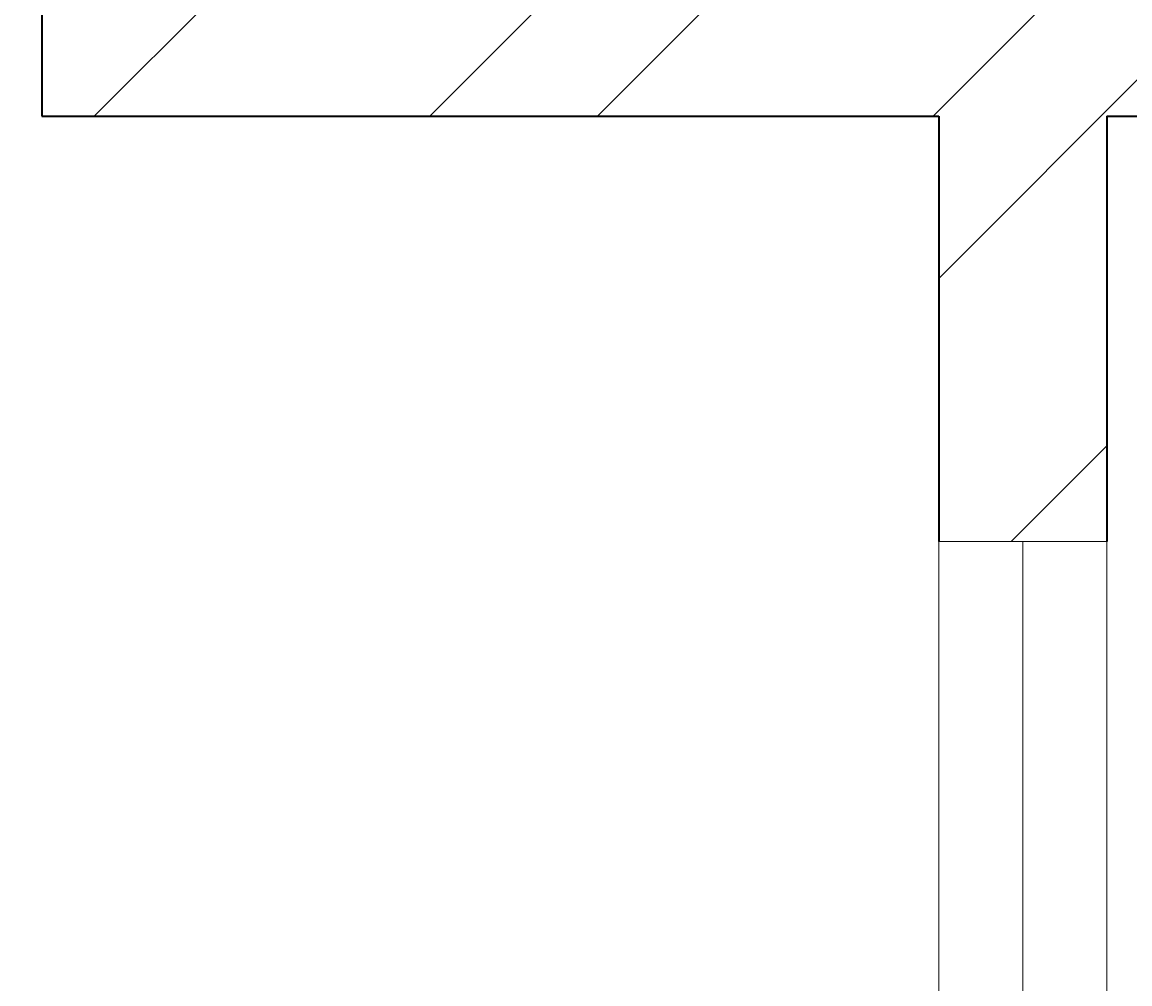
# Model space of a CAD drawing. Units: inches. Extents: x 1885 to 2748, y 783 to 2421.
# Tile 69 of 117: x 1992 to 2022, y 2047 to 2073. Entities that reach past the tile are written whole.
import ezdxf

# ---------------------------------------------------------------- set-up
doc = ezdxf.new("R2010")
doc.units = ezdxf.units.IN
for name, color, linetype, lineweight in [('A-ANNO-DIMS', 2, 'Continuous', 18), ('A-GLAZ', 181, 'Continuous', 18), ('A-WALL', 7, 'Continuous', 35)]:
    doc.layers.add(name, color=color, linetype=linetype, lineweight=lineweight)
doc.layers.add('A-WALL-PATT', color=85, linetype='Continuous', lineweight=13, true_color=0x58ba48)
doc.styles.get("Standard").update_dxf_attribs({"font": 'arial.ttf'})
doc.dimstyles.get("Standard").update_dxf_attribs({"dimtxt": 0.18, "dimasz": 0.18, "dimexe": 0.18, "dimexo": 0.0625, "dimgap": 0.09, "dimtad": 0, "dimtih": 1, "dimtoh": 1, "dimdec": 4, "dimzin": 0, "dimdsep": 46, "dimtxsty": 'Standard', "dimcen": 0.09, "dimadec": 0, "dimazin": 0, "dimtfac": 1, "dimtdec": 4, "dimtofl": 0, "dimtmove": 0, "dimatfit": 3, "dimfxl": 1, "dimtolj": 1, "dimtzin": 0, "dimarcsym": 0})

# ---------------------------------------------------------------- blocks, each defined once
blk = doc.blocks.new('*D48')
at = {"layer": 'A-ANNO-DIMS', "color": 0, "lineweight": -2, "transparency": 16777216}
for p, q in [((1980.711, 2348.006), (1902.844, 2348.006)), ((1903.024, 2347.826), (1903.024, 2114.937)), ((1903.024, 1881.686), (1903.024, 2114.574)), ((2016.711, 1881.506), (1902.844, 1881.506))]:
    blk.add_line(p, q, dxfattribs=at)
at = {"layer": 'A-ANNO-DIMS', "color": 0, "transparency": 16777216}
for points in [[(1902.994, 2347.826), (1903.054, 2347.826), (1903.024, 2348.006)], [(1902.994, 1881.686), (1903.054, 1881.686), (1903.024, 1881.506)]]:
    blk.add_solid(points, dxfattribs=at)
at = {"layer": 'Defpoints', "color": 0, "transparency": 16777216}
for p in [(1903.024, 2348.006), (1980.774, 2348.006), (2016.774, 1881.506)]:
    blk.add_point(p, dxfattribs=at)
at = {"layer": 'A-ANNO-DIMS', "color": 0, "transparency": 16777216, "insert": (1903.024, 2114.756), "char_height": 0.18, "attachment_point": 5}
blk.add_mtext('\\A1;466.5', dxfattribs=at)

msp = doc.modelspace()

# ---------------------------------------------------------------- hatches: boundary and pattern name
at = {"layer": 'A-WALL-PATT'}
h = msp.add_hatch(dxfattribs=at)
h.set_pattern_fill('ANSI32', color=256)
h.paths.add_polyline_path([(2007.772, 2318.006), (1980.774, 2318.006), (1980.774, 2281.215), (1985.274, 2281.215), (1985.274, 2313.506), (2007.772, 2313.506), (2007.772, 2315.756)])
h.paths.add_polyline_path([(2094.324, 2318.006), (2067.772, 2318.006), (2067.772, 2313.506), (2094.324, 2313.506), (2094.324, 2315.756)])
h.paths.add_polyline_path([(2131.367, 2315.756), (2131.367, 2318.006), (2131.189, 2318.006), (2112.609, 2318.006), (2112.609, 2313.506), (2117.274, 2313.506), (2117.274, 2255.201), (2121.774, 2255.201), (2121.774, 2313.506), (2131.367, 2313.506)])
h.paths.add_polyline_path([(2190.512, 2318.006), (2155.367, 2318.006), (2155.367, 2313.506), (2169.774, 2313.506), (2169.774, 2229.506), (2121.774, 2229.506), (2121.774, 2233.451), (2119.524, 2233.451), (2117.274, 2233.451), (2117.274, 2201.101), (2121.774, 2201.101), (2121.774, 2225.006), (2169.774, 2225.006), (2169.774, 2165.006), (2306.274, 2165.006), (2306.274, 2066.006), (2310.774, 2066.006), (2344.274, 2066.006), (2486.274, 2066.006), (2486.274, 1886.006), (2483.02, 1886.006), (2483.02, 1881.506), (2486.274, 1881.506), (2486.274, 1880.678), (2490.774, 1880.678), (2490.774, 2070.506), (2344.274, 2070.506), (2310.774, 2070.506), (2310.774, 2165.006), (2310.774, 2173.636), (2308.524, 2173.636), (2306.274, 2173.636), (2306.274, 2169.506), (2174.274, 2169.506), (2174.274, 2313.506), (2190.512, 2313.506), (2190.512, 2315.756)])
h.paths.add_polyline_path([(1985.274, 2221.215), (1980.774, 2221.215), (1980.774, 2165.006), (1992.774, 2165.006), (1992.774, 2141.927), (1997.274, 2141.927), (1997.274, 2165.006), (2117.274, 2165.006), (2117.274, 2163.126), (2121.774, 2163.126), (2121.774, 2172.734), (2119.524, 2172.734), (2117.274, 2172.734), (2117.274, 2169.506), (1985.274, 2169.506)])
h.paths.add_polyline_path([(1997.274, 2105.927), (1992.774, 2105.927), (1992.774, 2070.506), (2016.774, 2070.506), (2016.774, 2059.123), (2019.024, 2059.123), (2021.274, 2059.123), (2021.274, 2070.506), (2117.274, 2070.506), (2117.274, 2022.506), (2114.423, 2022.506), (2114.423, 2018.006), (2123.627, 2018.006), (2123.627, 2020.256), (2123.627, 2022.506), (2121.774, 2022.506), (2121.774, 2142.587), (2119.524, 2142.587), (2117.274, 2142.587), (2117.274, 2075.006), (1997.274, 2075.006)])
h.paths.add_polyline_path([(2092.029, 2020.256), (2092.029, 2022.506), (2021.274, 2022.506), (2021.274, 2035.123), (2016.774, 2035.123), (2016.774, 2018.006), (2016.774, 1978.784), (2021.274, 1978.784), (2021.274, 2018.006), (2092.029, 2018.006)])
h.paths.add_polyline_path([(2260.938, 2022.506), (2153.105, 2022.506), (2153.105, 2020.256), (2153.105, 2018.006), (2155.274, 2018.006), (2155.274, 1886.006), (2107.629, 1886.006), (2107.629, 1881.506), (2182.911, 1881.506), (2182.911, 1883.756), (2182.911, 1886.006), (2159.774, 1886.006), (2159.774, 2018.006), (2260.938, 2018.006), (2260.938, 2020.256)])
h.paths.add_polyline_path([(2047.629, 1883.756), (2047.629, 1886.006), (2021.274, 1886.006), (2021.274, 1918.784), (2019.024, 1918.784), (2016.774, 1918.784), (2016.774, 1881.506), (2047.629, 1881.506)])
h.paths.add_polyline_path([(2306.361, 1883.756), (2306.361, 1886.006), (2296.274, 1886.006), (2296.274, 1982.006), (2316.535, 1982.006), (2316.535, 1984.256), (2316.535, 1986.506), (2296.274, 1986.506), (2296.274, 2022.506), (2289.276, 2022.506), (2289.276, 2018.006), (2291.774, 2018.006), (2291.774, 1886.006), (2242.911, 1886.006), (2242.911, 1881.506), (2306.361, 1881.506)], flags=17)
h.paths.add_polyline_path([(1985.274, 1843.006), (2021.6, 1843.006), (2021.534, 1845.441), (2021.477, 1847.506), (1980.774, 1847.506), (1980.774, 1809.446), (1985.274, 1809.446)])
h.paths.add_polyline_path([(2131.482, 1845.256), (2131.482, 1847.506), (2081.534, 1847.506), (2081.534, 1843.006), (2117.274, 1843.006), (2117.274, 1784.147), (2119.524, 1784.147), (2121.774, 1784.147), (2121.774, 1843.006), (2131.482, 1843.006)])
h.paths.add_polyline_path([(2203.886, 1847.506), (2155.482, 1847.506), (2155.482, 1843.006), (2169.774, 1843.006), (2169.774, 1759.006), (2121.774, 1759.006), (2121.774, 1761.457), (2117.274, 1761.457), (2117.274, 1730.429), (2121.774, 1730.429), (2121.774, 1754.506), (2177.421, 1754.506), (2177.421, 1756.756), (2177.421, 1759.006), (2174.274, 1759.006), (2174.274, 1843.006), (2203.886, 1843.006)])
h.paths.add_polyline_path([(2335.554, 1845.256), (2335.554, 1847.506), (2239.886, 1847.506), (2239.886, 1843.006), (2306.274, 1843.006), (2306.274, 1759.006), (2199.486, 1759.006), (2199.486, 1754.506), (2310.774, 1754.506), (2310.774, 1843.006), (2335.554, 1843.006)])
h.paths.add_polyline_path([(2348.774, 2022.506), (2344.274, 2022.506), (2344.274, 1986.506), (2341.681, 1986.506), (2341.681, 1982.006), (2344.274, 1982.006), (2344.274, 1886.006), (2330.361, 1886.006), (2330.361, 1881.506), (2361.627, 1881.506), (2361.627, 1883.756), (2361.627, 1886.006), (2348.774, 1886.006)], flags=17)
h.paths.add_polyline_path([(2283.251, 2315.756), (2283.251, 2318.006), (2238.512, 2318.006), (2238.512, 2313.506), (2283.251, 2313.506)], flags=17)
h.paths.add_polyline_path([(2363.274, 2348.006), (2388.677, 2348.006), (2388.677, 2350.256), (2388.677, 2352.506), (2358.774, 2352.506), (2358.774, 2348.006), (2358.774, 2318.006), (2344.481, 2318.006), (2344.481, 2313.506), (2358.774, 2313.506), (2358.774, 2229.506), (2310.774, 2229.506), (2310.774, 2231.952), (2306.274, 2231.952), (2306.274, 2205.611), (2310.774, 2205.611), (2310.774, 2225.006), (2358.774, 2225.006), (2358.774, 2211.506), (2452.329, 2211.506), (2452.329, 2213.756), (2452.329, 2216.006), (2363.274, 2216.006), (2363.274, 2318.006)])
h.paths.add_polyline_path([(2310.774, 2313.506), (2320.481, 2313.506), (2320.481, 2315.756), (2320.481, 2318.006), (2302.728, 2318.006), (2302.728, 2313.506), (2306.274, 2313.506), (2306.274, 2251.076), (2310.774, 2251.076)], flags=17)
h.paths.add_polyline_path([(2490.774, 2352.506), (2486.274, 2352.506), (2448.677, 2352.506), (2448.677, 2348.006), (2486.274, 2348.006), (2486.274, 2318.006), (2486.274, 2216.006), (2481.78, 2216.006), (2481.78, 2211.506), (2486.274, 2211.506), (2486.274, 2165.006), (2493.289, 2165.006), (2493.289, 2167.256), (2493.289, 2169.506), (2490.774, 2169.506), (2490.774, 2313.506), (2494.429, 2313.506), (2494.429, 2318.006), (2490.774, 2318.006)])
h.paths.add_polyline_path([(2534.653, 2318.006), (2515.691, 2318.006), (2515.691, 2313.506), (2534.653, 2313.506), (2534.653, 2315.756)])
h.paths.add_polyline_path([(2618.274, 2318.006), (2594.653, 2318.006), (2594.653, 2313.506), (2613.774, 2313.506), (2613.774, 2281.706), (2618.274, 2281.706)])
h.paths.add_polyline_path([(2618.274, 2221.706), (2613.774, 2221.706), (2613.774, 2169.506), (2554.019, 2169.506), (2554.019, 2165.006), (2613.774, 2165.006), (2613.774, 2152.878), (2618.274, 2152.878)])
h.paths.add_polyline_path([(2618.274, 2128.878), (2616.024, 2128.878), (2613.774, 2128.878), (2613.774, 2117.006), (2529.774, 2117.006), (2529.774, 2165.006), (2532.848, 2165.006), (2532.848, 2169.506), (2522.867, 2169.506), (2522.867, 2165.006), (2525.274, 2165.006), (2525.274, 2117.006), (2525.274, 2112.506), (2525.274, 2108.576), (2529.774, 2108.576), (2529.774, 2112.506), (2613.774, 2112.506), (2613.774, 2080.19), (2618.274, 2080.19)])
h.paths.add_polyline_path([(2618.274, 2044.19), (2616.024, 2044.19), (2613.774, 2044.19), (2613.774, 2015.506), (2529.774, 2015.506), (2529.774, 2088.582), (2527.524, 2088.582), (2525.274, 2088.582), (2525.274, 2011.006), (2613.774, 2011.006), (2613.774, 1956.755), (2618.274, 1956.755)])
h.paths.add_polyline_path([(2618.274, 1881.506), (2618.274, 1896.755), (2613.774, 1896.755), (2613.774, 1881.506), (2613.774, 1847.506), (2592.715, 1847.506), (2592.715, 1843.006), (2613.774, 1843.006), (2613.774, 1765.006), (2613.774, 1760.506), (2609.621, 1760.506), (2609.621, 1756.006), (2613.774, 1756.006), (2613.774, 1660.006), (2608.544, 1660.006), (2608.544, 1655.506), (2613.774, 1655.506), (2613.774, 1508.158), (2618.274, 1508.158)])
h.paths.add_polyline_path([(2565.774, 1843.006), (2568.997, 1843.006), (2568.997, 1847.506), (2490.774, 1847.506), (2490.774, 1849.7), (2488.524, 1849.7), (2486.274, 1849.7), (2486.274, 1847.506), (2477.274, 1847.506), (2477.274, 1838.506), (2477.274, 1821.493), (2486.274, 1821.493), (2486.274, 1838.506), (2561.274, 1838.506), (2561.274, 1765.006), (2486.274, 1765.006), (2486.274, 1786.157), (2477.274, 1786.157), (2477.274, 1765.006), (2477.274, 1756.006), (2486.274, 1756.006), (2565.774, 1756.006), (2585.621, 1756.006), (2585.621, 1758.256), (2585.621, 1760.506), (2565.774, 1760.506), (2565.774, 1765.006)])
h.paths.add_polyline_path([(2486.274, 1651.006), (2561.274, 1651.006), (2561.274, 1567.006), (2486.274, 1567.006), (2486.274, 1591.321), (2477.274, 1591.321), (2477.274, 1567.006), (2477.274, 1558.006), (2477.274, 1555.439), (2481.774, 1555.439), (2481.774, 1558.006), (2568.653, 1558.006), (2568.653, 1560.256), (2568.653, 1562.506), (2565.774, 1562.506), (2565.774, 1655.506), (2584.544, 1655.506), (2584.544, 1657.756), (2584.544, 1660.006), (2565.774, 1660.006), (2486.274, 1660.006), (2477.274, 1660.006), (2477.274, 1651.006), (2477.274, 1632.989), (2486.274, 1632.989)])
h.paths.add_polyline_path([(2449.967, 1883.756), (2449.967, 1886.006), (2421.627, 1886.006), (2421.627, 1881.506), (2449.967, 1881.506)], flags=17)
h.paths.add_polyline_path([(2447.274, 1847.506), (2395.554, 1847.506), (2395.554, 1843.006), (2442.774, 1843.006), (2442.774, 1809.27), (2447.274, 1809.27)])
h.paths.add_polyline_path([(1985.274, 1749.446), (1980.774, 1749.446), (1980.774, 1694.504), (1985.274, 1694.504), (1985.274, 1694.506), (1986.897, 1694.506), (1986.897, 1697.78), (1986.897, 1699.006), (1985.274, 1699.006)])
h.paths.add_polyline_path([(2152.774, 1699.006), (2121.774, 1699.006), (2121.774, 1703.668), (2119.524, 1703.668), (2117.274, 1703.668), (2117.274, 1699.006), (2009.219, 1699.006), (2009.219, 1694.506), (2148.274, 1694.506), (2148.274, 1692.631), (2152.774, 1692.631)])
h.paths.add_polyline_path([(2016.274, 1694.506), (2011.774, 1694.506), (2011.774, 1558.006), (2040.806, 1558.006), (2040.806, 1560.256), (2040.806, 1562.506), (2016.274, 1562.506)])
h.paths.add_polyline_path([(2152.774, 1663.017), (2150.524, 1663.017), (2148.274, 1663.017), (2148.274, 1562.506), (2100.806, 1562.506), (2100.806, 1558.006), (2165.119, 1558.006), (2165.119, 1560.256), (2165.119, 1562.506), (2152.774, 1562.506), (2152.774, 1610.506), (2224.774, 1610.506), (2224.774, 1607.99), (2229.274, 1607.99), (2229.274, 1615.006), (2152.774, 1615.006)])
h.paths.add_polyline_path([(2238.613, 1560.256), (2238.613, 1562.506), (2229.274, 1562.506), (2229.274, 1588.756), (2227.024, 1588.763), (2224.774, 1588.771), (2224.774, 1562.506), (2189.119, 1562.506), (2189.119, 1558.006), (2238.613, 1558.006)])
h.paths.add_polyline_path([(2336.024, 1560.256), (2336.024, 1562.506), (2310.774, 1562.506), (2310.774, 1656.347), (2308.524, 1656.347), (2306.274, 1656.347), (2306.274, 1562.506), (2286.613, 1562.506), (2286.613, 1558.006), (2336.024, 1558.006)])
h.paths.add_polyline_path([(2447.274, 1690.968), (2445.024, 1690.968), (2442.774, 1690.968), (2442.774, 1687.006), (2306.274, 1687.006), (2306.274, 1680.75), (2310.774, 1680.75), (2310.774, 1682.506), (2442.774, 1682.506), (2442.774, 1562.506), (2396.024, 1562.506), (2396.024, 1558.006), (2447.274, 1558.006)])
h.paths.add_polyline_path([(2447.274, 1749.27), (2445.024, 1749.27), (2442.774, 1749.27), (2442.774, 1717.232), (2447.274, 1717.232)])
h.paths.add_polyline_path([(2044.674, 1521.756), (2044.674, 1524.006), (2007.274, 1524.006), (2007.274, 1503.49), (2009.524, 1503.49), (2011.774, 1503.49), (2011.774, 1519.506), (2044.674, 1519.506)])
h.paths.add_polyline_path([(2177.969, 1521.756), (2177.969, 1524.006), (2104.674, 1524.006), (2104.674, 1519.506), (2145.774, 1519.506), (2145.774, 1387.506), (2143.37, 1387.506), (2143.37, 1383.006), (2251.585, 1383.006), (2251.585, 1385.256), (2251.585, 1387.506), (2150.274, 1387.506), (2150.274, 1519.506), (2177.969, 1519.506)])
h.paths.add_polyline_path([(2298.704, 1524.006), (2237.969, 1524.006), (2237.969, 1519.506), (2282.274, 1519.506), (2282.274, 1387.506), (2279.683, 1387.506), (2279.683, 1383.006), (2286.774, 1383.006), (2286.774, 1419.006), (2312.451, 1419.006), (2312.451, 1421.256), (2312.451, 1423.506), (2286.774, 1423.506), (2286.774, 1519.506), (2298.704, 1519.506), (2298.704, 1521.722)], flags=17)
h.paths.add_polyline_path([(2361.897, 1521.756), (2361.897, 1524.006), (2322.704, 1524.006), (2322.704, 1519.506), (2334.774, 1519.506), (2334.774, 1423.506), (2331.93, 1423.506), (2331.93, 1419.006), (2334.774, 1419.006), (2334.774, 1387.506), (2334.774, 1383.228), (2339.274, 1383.228), (2339.274, 1387.506), (2339.274, 1519.506), (2361.897, 1519.506)], flags=17)
h.paths.add_polyline_path([(2447.274, 1521.756), (2447.274, 1524.006), (2421.897, 1524.006), (2421.897, 1519.506), (2447.274, 1519.506)], flags=17)
h.paths.add_polyline_path([(2481.774, 1529.6), (2479.524, 1529.6), (2477.274, 1529.6), (2477.274, 1524.006), (2474.489, 1524.006), (2474.489, 1519.506), (2477.274, 1519.506), (2477.274, 1334.506), (2296.774, 1334.506), (2296.774, 1240.506), (2160.274, 1240.506), (2160.274, 1180.506), (2112.274, 1180.506), (2112.274, 1207.692), (2110.024, 1207.692), (2107.774, 1207.692), (2107.774, 1171.609), (2112.274, 1171.609), (2112.274, 1176.006), (2160.274, 1176.006), (2160.274, 1092.006), (2144.221, 1092.006), (2144.221, 1087.506), (2189.497, 1087.506), (2189.497, 1089.756), (2189.497, 1092.006), (2164.774, 1092.006), (2164.774, 1236.006), (2296.774, 1236.006), (2296.774, 1231.912), (2301.274, 1231.912), (2301.274, 1330.006), (2481.774, 1330.006), (2481.774, 1387.506)])
h.paths.add_polyline_path([(2618.274, 1448.158), (2613.774, 1448.158), (2613.774, 1382.506), (2529.774, 1382.506), (2525.274, 1382.506), (2525.274, 1307.062), (2529.774, 1307.062), (2529.774, 1378.006), (2613.774, 1378.006), (2613.774, 1354.988), (2618.274, 1354.988)])
h.paths.add_polyline_path([(2618.274, 1318.988), (2613.774, 1318.988), (2613.774, 1281.006), (2529.774, 1281.006), (2529.774, 1283.786), (2527.524, 1283.786), (2525.274, 1283.786), (2525.274, 1228.506), (2516.794, 1228.506), (2516.794, 1224.006), (2533.484, 1224.006), (2533.484, 1226.256), (2533.484, 1228.506), (2529.774, 1228.506), (2529.774, 1276.506), (2613.774, 1276.506), (2613.774, 1266.02), (2618.274, 1266.02)])
h.paths.add_polyline_path([(2618.274, 1134.964), (2613.774, 1134.964), (2613.774, 1092.006), (2594.545, 1092.006), (2594.545, 1087.506), (2618.274, 1087.506)])
h.paths.add_polyline_path([(2534.545, 1092.006), (2509.765, 1092.006), (2509.765, 1087.506), (2534.545, 1087.506), (2534.545, 1089.756)])
h.paths.add_polyline_path([(2481.274, 1224.006), (2484.117, 1224.006), (2484.117, 1226.256), (2484.117, 1228.506), (2476.774, 1228.506), (2476.774, 1198.506), (2471.61, 1198.506), (2471.61, 1194.006), (2476.774, 1194.006), (2476.774, 1062.006), (2436.894, 1062.006), (2436.894, 1057.506), (2476.774, 1057.506), (2481.274, 1057.506), (2481.274, 1062.006), (2481.274, 1087.506), (2485.354, 1087.506), (2485.354, 1089.756), (2485.354, 1092.006), (2481.274, 1092.006), (2481.274, 1117.506)])
h.paths.add_polyline_path([(2439.898, 1198.506), (2349.274, 1198.506), (2349.274, 1194.006), (2349.274, 1180.506), (2301.274, 1180.506), (2301.274, 1201.896), (2299.024, 1201.896), (2296.774, 1201.896), (2296.774, 1172.335), (2299.024, 1172.335), (2301.274, 1172.335), (2301.274, 1176.006), (2349.274, 1176.006), (2349.274, 1092.006), (2334.452, 1092.006), (2334.452, 1087.506), (2349.274, 1087.506), (2349.274, 1057.506), (2353.774, 1057.506), (2376.894, 1057.506), (2376.894, 1059.756), (2376.894, 1062.006), (2353.774, 1062.006), (2353.774, 1087.506), (2353.774, 1180.506), (2353.774, 1194.006), (2439.898, 1194.006), (2439.898, 1196.256)])
h.paths.add_polyline_path([(2270.596, 1089.756), (2270.596, 1092.006), (2249.497, 1092.006), (2249.497, 1087.506), (2270.596, 1087.506)], flags=17)
h.paths.add_polyline_path([(2310.452, 1092.006), (2301.274, 1092.006), (2301.274, 1153.292), (2296.774, 1153.292), (2296.774, 1092.006), (2293.786, 1092.006), (2293.786, 1087.506), (2310.452, 1087.506), (2310.452, 1089.756)], flags=17)
h.paths.add_polyline_path([(2112.274, 1150.328), (2110.024, 1150.328), (2107.774, 1150.328), (2107.774, 1092.006), (2104.465, 1092.006), (2104.465, 1087.506), (2120.221, 1087.506), (2120.221, 1089.756), (2120.221, 1092.006), (2112.274, 1092.006)])
h.paths.add_polyline_path([(2082.172, 1092.006), (2058.144, 1092.006), (2058.144, 1087.506), (2082.172, 1087.506), (2082.172, 1089.756)])
h.paths.add_polyline_path([(1975.774, 1145.638), (1971.274, 1145.638), (1971.274, 1087.506), (1980.774, 1087.506), (1998.144, 1087.506), (1998.144, 1089.756), (1998.144, 1092.006), (1985.274, 1092.006), (1975.774, 1092.006)])
h.paths.add_polyline_path([(2112.274, 1244.385), (2110.024, 1244.385), (2107.774, 1244.385), (2107.774, 1240.506), (1992.274, 1240.506), (1992.274, 1271.008), (1987.774, 1271.008), (1987.774, 1240.506), (1980.774, 1240.506), (1975.774, 1240.506), (1971.274, 1240.506), (1971.274, 1205.638), (1975.774, 1205.638), (1975.774, 1236.006), (2107.774, 1236.006), (2107.774, 1233.444), (2112.274, 1233.444), (2112.274, 1236.006)])
h.paths.add_polyline_path([(2112.274, 1383.006), (2114.783, 1383.006), (2114.783, 1385.256), (2114.783, 1387.506), (2102.476, 1387.506), (2102.476, 1383.006), (2107.774, 1383.006), (2107.774, 1335.006), (2011.774, 1335.006), (2011.774, 1349.939), (2007.274, 1349.939), (2007.274, 1335.006), (1987.774, 1335.006), (1987.774, 1330.506), (1987.774, 1307.008), (1992.274, 1307.008), (1992.274, 1330.506), (2007.274, 1330.506), (2107.774, 1330.506), (2107.774, 1264.711), (2112.274, 1264.711)])
h.paths.add_polyline_path([(2077.857, 1387.506), (2011.774, 1387.506), (2011.774, 1390.036), (2009.524, 1390.036), (2007.274, 1390.036), (2007.274, 1373.939), (2011.774, 1373.939), (2011.774, 1383.006), (2077.857, 1383.006)])
h.paths.add_polyline_path([(2011.774, 1443.49), (2007.274, 1443.49), (2007.274, 1410.248), (2011.774, 1410.248)])

# ---------------------------------------------------------------- linework, layer by layer
at = {"layer": 'A-GLAZ'}
for p, q in [((2021.274, 2059.123), (2016.774, 2059.123)), ((2016.774, 2059.123), (2019.024, 2059.123)), ((2016.774, 2059.123), (2016.774, 2035.123)), ((2019.024, 2059.123), (2019.024, 2035.123)), ((2021.274, 2035.123), (2021.274, 2059.123))]:
    msp.add_line(p, q, dxfattribs=at)
at = {"layer": 'A-WALL'}
for p, q in [((1992.774, 2105.927), (1992.774, 2070.506)), ((1992.774, 2070.506), (2016.774, 2070.506)), ((2016.774, 2070.506), (2016.774, 2059.123)), ((2021.274, 2070.506), (2021.274, 2059.123)), ((2021.274, 2070.506), (2117.274, 2070.506))]:
    msp.add_line(p, q, dxfattribs=at)

# ---------------------------------------------------------------- dimensions: what is measured, and where the dimension line sits
at = {"layer": 'A-ANNO-DIMS'}
dim = msp.add_linear_dim(base=(1903.024, 2348.006), p1=(2016.774, 1881.506), p2=(1980.774, 2348.006), angle=90, dimstyle='Standard', override={"dimdec": 1, "dimlfac": 1, "dimrnd": 0, "dimzin": 0, "dimdsep": 46, "dimlunit": 2}, dxfattribs=at)
dim.commit()
dim.dimension.update_dxf_attribs({"geometry": '*D48', "text_midpoint": (1903.024, 2114.756)})

doc.saveas('drawing.dxf')
